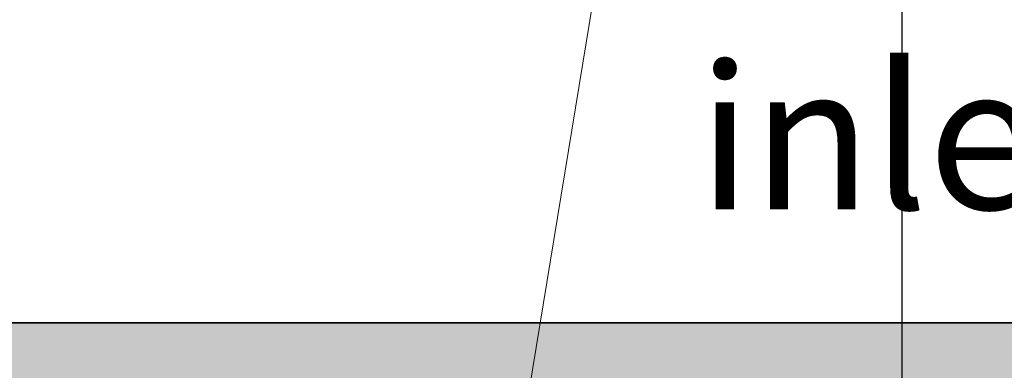
# Model space of a CAD drawing. Units: inches. Extents: x -1 to 292, y -3 to 199.
# Tile 31 of 52: x 146 to 181, y 118 to 130. Entities that reach past the tile are written whole.
import ezdxf

# ---------------------------------------------------------------- set-up
doc = ezdxf.new("R2010")
doc.units = ezdxf.units.IN
doc.header["$MEASUREMENT"] = 0
for name, color, linetype, lineweight in [('M-ANNO-LEAD', 2, 'Continuous', 18), ('M-ANNO-TEXT', 3, 'Continuous', 25), ('M-DIMS', 2, 'Continuous', 18), ('M-EQPM', 7, 'Continuous', 35), ('M-PATT', 8, 'Continuous', 13)]:
    doc.layers.add(name, color=color, linetype=linetype, lineweight=lineweight)
doc.styles.get("Standard").update_dxf_attribs({"font": 'arial.ttf'})
doc.dimstyles.get("Standard").update_dxf_attribs({"dimtxt": 0.18, "dimasz": 0.18, "dimexe": 0.18, "dimexo": 0.0625, "dimgap": 0.09, "dimtad": 0, "dimtih": 1, "dimtoh": 1, "dimdec": 4, "dimzin": 0, "dimdsep": 46, "dimtxsty": 'Standard', "dimcen": 0.09, "dimadec": 0, "dimazin": 0, "dimtfac": 1, "dimtdec": 4, "dimtofl": 0, "dimtmove": 0, "dimatfit": 3, "dimfxl": 1, "dimtolj": 1, "dimtzin": 0, "dimarcsym": 0})

# ---------------------------------------------------------------- blocks, each defined once
blk = doc.blocks.new('*D9')
at = {"layer": 'Defpoints', "color": 0, "transparency": 16777216}
for p in [(177.053, 174.363), (49.924, 99.774), (177.053, 99.774)]:
    blk.add_point(p, dxfattribs=at)
at = {"layer": 'M-DIMS', "color": 0, "lineweight": -2, "transparency": 16777216}
for p, q in [((49.924, 99.836), (49.924, 174.543)), ((50.104, 174.363), (113.033, 174.363)), ((176.873, 174.363), (113.943, 174.363)), ((177.053, 99.836), (177.053, 174.543))]:
    blk.add_line(p, q, dxfattribs=at)
at = {"layer": 'M-DIMS', "color": 0, "transparency": 16777216}
for points in [[(50.104, 174.393), (50.104, 174.333), (49.924, 174.363)], [(176.873, 174.393), (176.873, 174.333), (177.053, 174.363)]]:
    blk.add_solid(points, dxfattribs=at)
at = {"layer": 'M-DIMS', "color": 0, "transparency": 16777216, "insert": (113.488, 174.363), "char_height": 0.18, "attachment_point": 5}
blk.add_mtext('\\A1;127.13', dxfattribs=at)

msp = doc.modelspace()

# ---------------------------------------------------------------- hatches: boundary and pattern name
at = {"layer": 'M-PATT'}
h = msp.add_hatch(color=256, dxfattribs=at)
h.set_gradient(color1=(0, 127, 0), color2=(0, 127, 0), tint=1, name='CYLINDER')
h.paths.add_polyline_path([(164.5186, 119.2985), (129.9293, 119.2985), (129.9293, 117.2985), (164.1897, 117.2985)])
h.paths.add_polyline_path([(181.5897, 119.2985), (164.5186, 119.2985), (164.1897, 117.2985), (179.5897, 117.2985), (179.5897, 107.8518), (181.5897, 109.1506)])
h.paths.add_polyline_path([(181.5897, 109.1506), (179.5897, 107.8518), (179.5897, 36.2698), (198.4159, 36.2698), (198.4159, 38.2698), (181.5897, 38.2698)])
h.paths.add_polyline_path([(115.4883, 126.765), (111.4883, 126.765), (111.4883, 114.6589), (115.4883, 114.6589)])
h.paths.add_polyline_path([(123.408, 119.2985), (115.4883, 119.2985), (115.4883, 117.2985), (123.408, 117.2985)])
h.paths.add_polyline_path([(115.4883, 112.6589), (111.4883, 112.6589), (111.4883, 106.9941), (115.4883, 106.9941)])
h.paths.add_polyline_path([(120.9032, 106.9941), (106.0735, 106.9941), (106.0735, 105.9941), (120.9032, 105.9941)])
h.paths.add_polyline_path([(236.4209, 117.5104), (234.9209, 117.5104), (234.9209, 97.1861), (236.4209, 97.1861)])
h.paths.add_polyline_path([(236.4209, 126.4904), (234.9209, 126.4904), (234.9209, 118.9331), (236.4209, 118.9331)])
h.paths.add_polyline_path([(244.9552, 125.7269), (242.9552, 125.7269), (242.9552, 116.8562), (244.9552, 116.8562)])
h.paths.add_polyline_path([(244.9552, 115.1721), (242.9552, 115.1721), (242.9552, 109.7385), (244.9552, 109.7385)])
h.paths.add_polyline_path([(248.4468, 109.7385), (239.4637, 109.7385), (239.4637, 109.4289), (248.4468, 109.4289)])

# ---------------------------------------------------------------- linework, layer by layer
at = {"layer": 'M-ANNO-LEAD'}
msp.add_line((162.951, 109.7655), (166.6813, 132.451), dxfattribs=at)
at = {"layer": 'M-EQPM'}
msp.add_lwpolyline([(129.9293, 119.2985), (181.5897, 119.2985), (181.5897, 38.2698)], dxfattribs=at)

# ---------------------------------------------------------------- texts
at = {"layer": 'M-ANNO-TEXT', "insert": (169.9729, 136.5612), "char_height": 5, "attachment_point": 1}
msp.add_mtext_dynamic_manual_height_columns('feed water inlet', width=47.899539, gutter_width=1, heights=[0], dxfattribs=at)

# ---------------------------------------------------------------- dimensions: what is measured, and where the dimension line sits
at = {"layer": 'M-DIMS'}
dim = msp.add_linear_dim(base=(177.0526, 174.3627), p1=(49.9241, 99.7735), p2=(177.0526, 99.7735), dimstyle='Standard', override={"dimdec": 2, "dimlfac": 1, "dimrnd": 0, "dimzin": 0, "dimdsep": 46, "dimlunit": 2}, dxfattribs=at)
dim.commit()
dim.dimension.update_dxf_attribs({"geometry": '*D9', "text_midpoint": (113.4883, 174.3627)})

doc.saveas('drawing.dxf')
